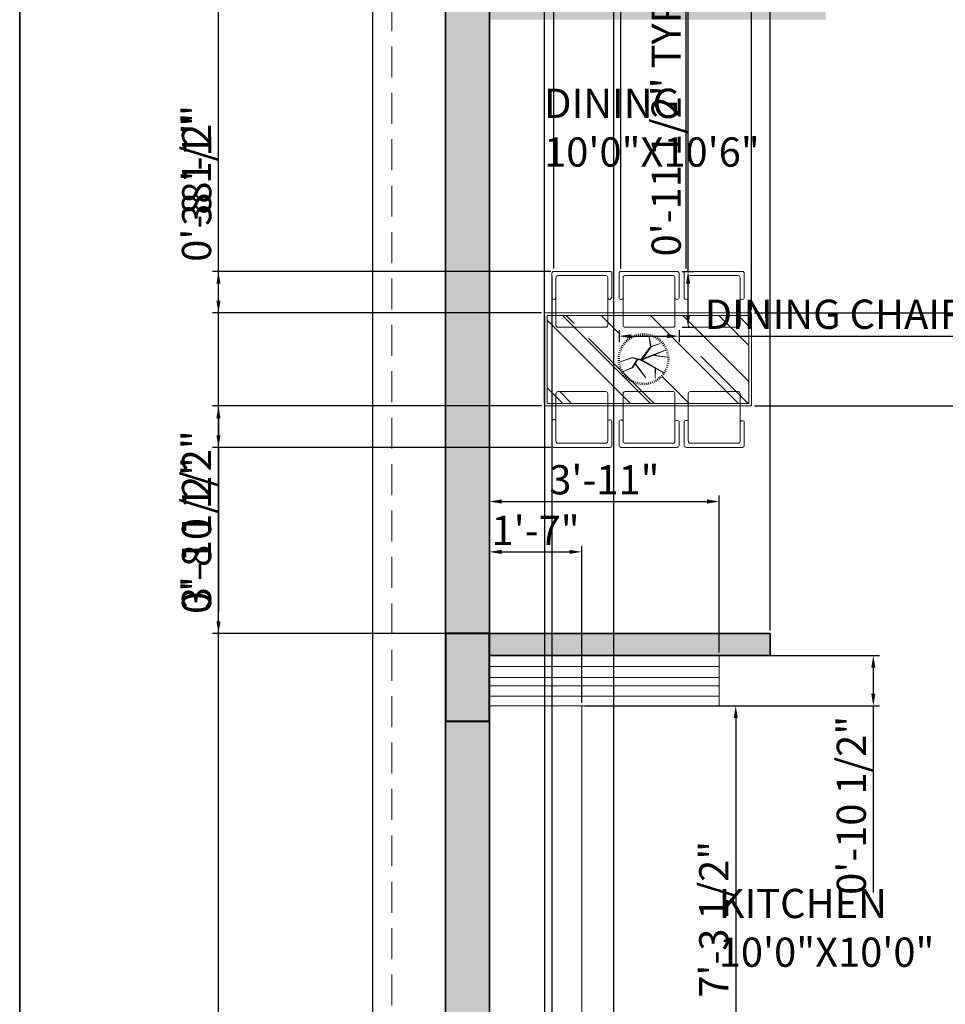
# Model space of a CAD drawing. Units: inches. Extents: x 2656 to 9931, y 1941 to 3068.
# Tile 2 of 46: x 2656 to 2846, y 2224 to 2426. Entities that reach past the tile are written whole.
import ezdxf

# ---------------------------------------------------------------- set-up
doc = ezdxf.new("R2010")
doc.units = ezdxf.units.IN
doc.linetypes.add('DASHED2', pattern=[9.525, 6.35, -3.175])
for name, color, linetype, lineweight in [('A-ANNO-DIMS', 2, 'Continuous', 18), ('A-ANNO-TTLB', 7, 'Continuous', 35), ('A-AREA-IDEN', 7, 'Continuous', 18), ('A-COLS', 7, 'Continuous', 40), ('A-COLS-PATT', 146, 'Continuous', 13), ('A-FLOR-CASE', 32, 'Continuous', 18), ('A-FLOR-OVHD', 252, 'DASHED2', 13), ('A-FURN', 8, 'Continuous', 13), ('A-FURN-PATT', 9, 'Continuous', 13), ('A-WALL', 7, 'Continuous', 35), ('A-WALL-PATT', 251, 'Continuous', 13), ('C-PROP', 7, 'Continuous', 25)]:
    doc.layers.add(name, color=color, linetype=linetype, lineweight=lineweight)
doc.styles.get("Standard").update_dxf_attribs({"font": 'arial.ttf'})
doc.dimstyles.new('ISO-25', dxfattribs={"dimtxt": 6, "dimasz": 2.5, "dimexe": 1.25, "dimexo": 0.625, "dimtad": 1, "dimdec": 0, "dimlunit": 3, "dimtxsty": 'Standard', "dimcen": 2.5, "dimadec": 0, "dimazin": 0, "dimtfac": 1, "dimtdec": 0, "dimtmove": 0, "dimatfit": 3, "dimfxl": 1, "dimarcsym": 0})

# ---------------------------------------------------------------- blocks, each defined once
blk = doc.blocks.new('CHAIR-DINING')
for p, q in [((-0.04, 6.08), (-0.04, 11.03)), ((0.34, 11.42), (11.9, 11.42)), ((0.81, 10.18), (0.81, 0.37)), ((1.19, 10.57), (11.05, 10.57)), ((11.43, 10.18), (11.43, 0.37)), ((12.28, 11.03), (12.28, 6.08)), ((0.34, 5.7), (0.43, 5.7)), ((11.82, 5.7), (11.9, 5.7)), ((1.19, -0.02), (11.05, -0.02))]:
    blk.add_line(p, q)
for centre, start, end in [((0.34, 11.03), 90, 180), ((1.19, 10.18), 90, 180), ((11.05, 10.18), 0, 90), ((11.9, 11.03), 0, 90), ((0.34, 6.08), 180, 270), ((0.43, 6.08), 270, 0), ((11.82, 6.08), 180, 270), ((11.9, 6.08), 270, 0), ((1.19, 0.37), 180, 270), ((11.05, 0.37), 270, 0)]:
    blk.add_arc(centre, 0.382, start, end)
blk = doc.blocks.new('*D61')
at = {"layer": 'A-ANNO-DIMS', "color": 0, "lineweight": -2, "transparency": 16777216}
for p, q in [((2778.76, 2362.36), (2778.76, 2359.89)), ((2781.26, 2361.14), (2788.58, 2361.14)), ((2791.08, 2362.36), (2791.08, 2359.89)), ((2791.08, 2361.14), (2905.16, 2361.14))]:
    blk.add_line(p, q, dxfattribs=at)
at = {"layer": 'A-ANNO-DIMS', "color": 0, "transparency": 16777216}
for points in [[(2781.26, 2361.55), (2781.26, 2360.72), (2778.76, 2361.14)], [(2788.58, 2361.55), (2788.58, 2360.72), (2791.08, 2361.14)]]:
    blk.add_solid(points, dxfattribs=at)
at = {"layer": 'Defpoints', "color": 0, "transparency": 16777216}
for p in [(2778.76, 2362.98), (2791.08, 2362.98), (2791.08, 2361.14)]:
    blk.add_point(p, dxfattribs=at)
at = {"layer": 'A-ANNO-DIMS', "color": 0, "transparency": 16777216, "insert": (2849.37, 2364.86), "char_height": 6, "attachment_point": 5}
blk.add_mtext('DINING CHAIR 1\'-0 1/2" TYP.', dxfattribs=at)
blk = doc.blocks.new('*D62')
at = {"layer": 'A-ANNO-DIMS', "color": 0, "lineweight": -2, "transparency": 16777216}
for p, q in [((2792.93, 2374.42), (2792.93, 2433.38)), ((2791.71, 2374.42), (2794.18, 2374.42)), ((2792.93, 2365.48), (2792.93, 2371.92)), ((2791.71, 2362.98), (2794.18, 2362.98))]:
    blk.add_line(p, q, dxfattribs=at)
at = {"layer": 'A-ANNO-DIMS', "color": 0, "transparency": 16777216}
for points in [[(2792.52, 2371.92), (2793.35, 2371.92), (2792.93, 2374.42)], [(2792.52, 2365.48), (2793.35, 2365.48), (2792.93, 2362.98)]]:
    blk.add_solid(points, dxfattribs=at)
at = {"layer": 'Defpoints', "color": 0, "transparency": 16777216}
for p in [(2791.08, 2374.42), (2792.93, 2374.42), (2791.08, 2362.98)]:
    blk.add_point(p, dxfattribs=at)
at = {"layer": 'A-ANNO-DIMS', "color": 0, "transparency": 16777216, "insert": (2789.21, 2405.15), "char_height": 6, "attachment_point": 5, "rotation": 90}
blk.add_mtext('0\'-11 1/2" TYP.', dxfattribs=at)
blk = doc.blocks.new('*D113')
at = {"layer": 'A-ANNO-DIMS', "color": 0, "lineweight": -2, "transparency": 16777216}
for p, q in [((2752.16, 2300.73), (2752.16, 2674.45)), ((2809.77, 2300.73), (2809.77, 2674.45)), ((2754.66, 2673.2), (2807.27, 2673.2))]:
    blk.add_line(p, q, dxfattribs=at)
at = {"layer": 'A-ANNO-DIMS', "color": 0, "transparency": 16777216}
for points in [[(2754.66, 2673.62), (2754.66, 2672.78), (2752.16, 2673.2)], [(2807.27, 2673.62), (2807.27, 2672.78), (2809.77, 2673.2)]]:
    blk.add_solid(points, dxfattribs=at)
at = {"layer": 'Defpoints', "color": 0, "transparency": 16777216}
for p in [(2809.77, 2673.2), (2752.16, 2300.1), (2809.77, 2300.1)]:
    blk.add_point(p, dxfattribs=at)
at = {"layer": 'A-ANNO-DIMS', "color": 0, "transparency": 16777216, "insert": (2780.96, 2676.93), "char_height": 6, "attachment_point": 5}
blk.add_mtext('4\'-9 1/2"', dxfattribs=at)
blk = doc.blocks.new('*D114')
at = {"layer": 'A-ANNO-DIMS', "color": 0, "lineweight": -2, "transparency": 16777216}
for p, q in [((2809.77, 2300.73), (2809.77, 2674.45)), ((2851.88, 2300.73), (2851.88, 2674.45)), ((2812.27, 2673.2), (2849.38, 2673.2))]:
    blk.add_line(p, q, dxfattribs=at)
at = {"layer": 'A-ANNO-DIMS', "color": 0, "transparency": 16777216}
for points in [[(2812.27, 2673.62), (2812.27, 2672.78), (2809.77, 2673.2)], [(2849.38, 2673.62), (2849.38, 2672.78), (2851.88, 2673.2)]]:
    blk.add_solid(points, dxfattribs=at)
at = {"layer": 'Defpoints', "color": 0, "transparency": 16777216}
for p in [(2851.88, 2673.2), (2809.77, 2300.1), (2851.88, 2300.1)]:
    blk.add_point(p, dxfattribs=at)
at = {"layer": 'A-ANNO-DIMS', "color": 0, "transparency": 16777216, "insert": (2830.82, 2676.89), "char_height": 6, "attachment_point": 5}
blk.add_mtext('3\'-6"', dxfattribs=at)
blk = doc.blocks.new('*D116')
at = {"layer": 'A-ANNO-DIMS', "color": 0, "lineweight": -2, "transparency": 16777216}
for p, q in [((2752.16, 2296.23), (2752.16, 2328.45)), ((2799.34, 2296.23), (2799.34, 2328.45)), ((2754.66, 2327.2), (2796.84, 2327.2))]:
    blk.add_line(p, q, dxfattribs=at)
at = {"layer": 'A-ANNO-DIMS', "color": 0, "transparency": 16777216}
for points in [[(2754.66, 2327.62), (2754.66, 2326.78), (2752.16, 2327.2)], [(2796.84, 2327.62), (2796.84, 2326.78), (2799.34, 2327.2)]]:
    blk.add_solid(points, dxfattribs=at)
at = {"layer": 'Defpoints', "color": 0, "transparency": 16777216}
for p in [(2799.34, 2327.2), (2752.16, 2295.6), (2799.34, 2295.6)]:
    blk.add_point(p, dxfattribs=at)
at = {"layer": 'A-ANNO-DIMS', "color": 0, "transparency": 16777216, "insert": (2775.75, 2330.89), "char_height": 6, "attachment_point": 5}
blk.add_mtext('3\'-11"', dxfattribs=at)
blk = doc.blocks.new('*D117')
at = {"layer": 'A-ANNO-DIMS', "color": 0, "lineweight": -2, "transparency": 16777216}
for p, q in [((2799.96, 2295.6), (2832.19, 2295.6)), ((2830.94, 2293.1), (2830.94, 2287.76)), ((2799.96, 2285.26), (2832.19, 2285.26)), ((2830.94, 2285.26), (2830.94, 2246.92))]:
    blk.add_line(p, q, dxfattribs=at)
at = {"layer": 'A-ANNO-DIMS', "color": 0, "transparency": 16777216}
for points in [[(2830.52, 2293.1), (2831.36, 2293.1), (2830.94, 2295.6)], [(2830.52, 2287.76), (2831.36, 2287.76), (2830.94, 2285.26)]]:
    blk.add_solid(points, dxfattribs=at)
at = {"layer": 'Defpoints', "color": 0, "transparency": 16777216}
for p in [(2799.34, 2295.6), (2799.34, 2285.26), (2830.94, 2285.26)]:
    blk.add_point(p, dxfattribs=at)
at = {"layer": 'A-ANNO-DIMS', "color": 0, "transparency": 16777216, "insert": (2827.21, 2264.84), "char_height": 6, "attachment_point": 5, "rotation": 90}
blk.add_mtext('0\'-10 1/2"', dxfattribs=at)
blk = doc.blocks.new('*D118')
at = {"layer": 'A-ANNO-DIMS', "color": 0, "lineweight": -2, "transparency": 16777216}
for p, q in [((2752.16, 2285.89), (2752.16, 2318.11)), ((2771.11, 2285.89), (2771.11, 2318.11)), ((2754.66, 2316.86), (2768.61, 2316.86))]:
    blk.add_line(p, q, dxfattribs=at)
at = {"layer": 'A-ANNO-DIMS', "color": 0, "transparency": 16777216}
for points in [[(2754.66, 2317.28), (2754.66, 2316.45), (2752.16, 2316.86)], [(2768.61, 2317.28), (2768.61, 2316.45), (2771.11, 2316.86)]]:
    blk.add_solid(points, dxfattribs=at)
at = {"layer": 'Defpoints', "color": 0, "transparency": 16777216}
for p in [(2771.11, 2316.86), (2752.16, 2285.26), (2771.11, 2285.26)]:
    blk.add_point(p, dxfattribs=at)
at = {"layer": 'A-ANNO-DIMS', "color": 0, "transparency": 16777216, "insert": (2761.63, 2320.5), "char_height": 6, "attachment_point": 5}
blk.add_mtext('1\'-7"', dxfattribs=at)
blk = doc.blocks.new('*D119')
at = {"layer": 'A-ANNO-DIMS', "color": 0, "lineweight": -2, "transparency": 16777216}
for p, q in [((2771.73, 2285.26), (2803.96, 2285.26)), ((2802.71, 2282.76), (2802.71, 2200.13)), ((2771.73, 2197.63), (2803.96, 2197.63))]:
    blk.add_line(p, q, dxfattribs=at)
at = {"layer": 'A-ANNO-DIMS', "color": 0, "transparency": 16777216}
for points in [[(2802.29, 2282.76), (2803.12, 2282.76), (2802.71, 2285.26)], [(2802.29, 2200.13), (2803.12, 2200.13), (2802.71, 2197.63)]]:
    blk.add_solid(points, dxfattribs=at)
at = {"layer": 'Defpoints', "color": 0, "transparency": 16777216}
for p in [(2771.11, 2285.26), (2771.11, 2197.63), (2802.71, 2197.63)]:
    blk.add_point(p, dxfattribs=at)
at = {"layer": 'A-ANNO-DIMS', "color": 0, "transparency": 16777216, "insert": (2798.98, 2241.45), "char_height": 6, "attachment_point": 5, "rotation": 90}
blk.add_mtext('7\'-3 1/2"', dxfattribs=at)
blk = doc.blocks.new('*D129')
at = {"layer": 'A-ANNO-DIMS', "color": 0, "lineweight": -2, "transparency": 16777216}
for p, q in [((2752.16, 2601.15), (2752.16, 2009.27)), ((2777.59, 2557.74), (2777.59, 2009.27)), ((2754.66, 2010.52), (2775.09, 2010.52)), ((2777.59, 2010.52), (2811.37, 2010.52))]:
    blk.add_line(p, q, dxfattribs=at)
at = {"layer": 'A-ANNO-DIMS', "color": 0, "transparency": 16777216}
for points in [[(2754.66, 2010.94), (2754.66, 2010.11), (2752.16, 2010.52)], [(2775.09, 2010.94), (2775.09, 2010.11), (2777.59, 2010.52)]]:
    blk.add_solid(points, dxfattribs=at)
at = {"layer": 'Defpoints', "color": 0, "transparency": 16777216}
for p in [(2752.16, 2601.77), (2777.59, 2558.37), (2777.59, 2010.52)]:
    blk.add_point(p, dxfattribs=at)
at = {"layer": 'A-ANNO-DIMS', "color": 0, "transparency": 16777216, "insert": (2795.73, 2014.25), "char_height": 6, "attachment_point": 5}
blk.add_mtext('2\'-1 1/2"', dxfattribs=at)
blk = doc.blocks.new('*D132')
at = {"layer": 'A-ANNO-DIMS', "color": 0, "lineweight": -2, "transparency": 16777216}
for p, q in [((2763.47, 2366.56), (2763.47, 2674.45)), ((2805.96, 2366.56), (2805.96, 2674.45)), ((2765.97, 2673.2), (2803.46, 2673.2))]:
    blk.add_line(p, q, dxfattribs=at)
at = {"layer": 'A-ANNO-DIMS', "color": 0, "transparency": 16777216}
for points in [[(2765.97, 2673.62), (2765.97, 2672.78), (2763.47, 2673.2)], [(2803.46, 2673.62), (2803.46, 2672.78), (2805.96, 2673.2)]]:
    blk.add_solid(points, dxfattribs=at)
at = {"layer": 'Defpoints', "color": 0, "transparency": 16777216}
for p in [(2805.96, 2673.2), (2763.47, 2365.93), (2805.96, 2365.93)]:
    blk.add_point(p, dxfattribs=at)
at = {"layer": 'A-ANNO-DIMS', "color": 0, "transparency": 16777216, "insert": (2784.72, 2676.93), "char_height": 6, "attachment_point": 5}
blk.add_mtext('3\'-6 1/2"', dxfattribs=at)
blk = doc.blocks.new('*D133')
at = {"layer": 'A-ANNO-DIMS', "color": 0, "lineweight": -2, "transparency": 16777216}
for p, q in [((2806.59, 2365.93), (3061.01, 2365.93)), ((3059.76, 2349.31), (3059.76, 2363.43)), ((2806.59, 2346.81), (3061.01, 2346.81))]:
    blk.add_line(p, q, dxfattribs=at)
at = {"layer": 'A-ANNO-DIMS', "color": 0, "transparency": 16777216}
for points in [[(3059.34, 2363.43), (3060.17, 2363.43), (3059.76, 2365.93)], [(3059.34, 2349.31), (3060.17, 2349.31), (3059.76, 2346.81)]]:
    blk.add_solid(points, dxfattribs=at)
at = {"layer": 'Defpoints', "color": 0, "transparency": 16777216}
for p in [(2805.96, 2365.93), (3059.76, 2365.93), (2805.96, 2346.81)]:
    blk.add_point(p, dxfattribs=at)
at = {"layer": 'A-ANNO-DIMS', "color": 0, "transparency": 16777216, "insert": (3056.12, 2356.37), "char_height": 6, "attachment_point": 5, "rotation": 90}
blk.add_mtext('1\'-7"', dxfattribs=at)
blk = doc.blocks.new('*D134')
at = {"layer": 'A-ANNO-DIMS', "color": 0, "lineweight": -2, "transparency": 16777216}
for p, q in [((2752.16, 2300.73), (2752.16, 2674.45)), ((2763.47, 2347.43), (2763.47, 2674.45)), ((2754.66, 2673.2), (2760.97, 2673.2)), ((2763.47, 2673.2), (2801.81, 2673.2))]:
    blk.add_line(p, q, dxfattribs=at)
at = {"layer": 'A-ANNO-DIMS', "color": 0, "transparency": 16777216}
for points in [[(2754.66, 2673.62), (2754.66, 2672.78), (2752.16, 2673.2)], [(2760.97, 2673.62), (2760.97, 2672.78), (2763.47, 2673.2)]]:
    blk.add_solid(points, dxfattribs=at)
at = {"layer": 'Defpoints', "color": 0, "transparency": 16777216}
for p in [(2763.47, 2673.2), (2763.47, 2346.81), (2752.16, 2300.1)]:
    blk.add_point(p, dxfattribs=at)
at = {"layer": 'A-ANNO-DIMS', "color": 0, "transparency": 16777216, "insert": (2783.89, 2676.93), "char_height": 6, "attachment_point": 5}
blk.add_mtext('0\'-11 1/2"', dxfattribs=at)
blk = doc.blocks.new('*D135')
at = {"layer": 'A-ANNO-DIMS', "color": 0, "lineweight": -2, "transparency": 16777216}
for p, q in [((2762.84, 2346.81), (2695.31, 2346.81)), ((2696.56, 2302.6), (2696.56, 2344.31)), ((2751.53, 2300.1), (2695.31, 2300.1))]:
    blk.add_line(p, q, dxfattribs=at)
at = {"layer": 'A-ANNO-DIMS', "color": 0, "transparency": 16777216}
for points in [[(2696.14, 2344.31), (2696.97, 2344.31), (2696.56, 2346.81)], [(2696.14, 2302.6), (2696.97, 2302.6), (2696.56, 2300.1)]]:
    blk.add_solid(points, dxfattribs=at)
at = {"layer": 'Defpoints', "color": 0, "transparency": 16777216}
for p in [(2696.56, 2346.81), (2763.47, 2346.81), (2752.16, 2300.1)]:
    blk.add_point(p, dxfattribs=at)
at = {"layer": 'A-ANNO-DIMS', "color": 0, "transparency": 16777216, "insert": (2692.83, 2323.45), "char_height": 6, "attachment_point": 5, "rotation": 90}
blk.add_mtext('3\'-10 1/2"', dxfattribs=at)
blk = doc.blocks.new('*D136')
at = {"layer": 'A-ANNO-DIMS', "color": 0, "lineweight": -2, "transparency": 16777216}
for p, q in [((2765.36, 2375.04), (2765.36, 2674.45)), ((2779.14, 2375.04), (2779.14, 2674.45)), ((2767.86, 2673.2), (2776.64, 2673.2)), ((2779.14, 2673.2), (2798.28, 2673.2))]:
    blk.add_line(p, q, dxfattribs=at)
at = {"layer": 'A-ANNO-DIMS', "color": 0, "transparency": 16777216}
for points in [[(2767.86, 2673.62), (2767.86, 2672.78), (2765.36, 2673.2)], [(2776.64, 2673.62), (2776.64, 2672.78), (2779.14, 2673.2)]]:
    blk.add_solid(points, dxfattribs=at)
at = {"layer": 'Defpoints', "color": 0, "transparency": 16777216}
for p in [(2779.14, 2673.2), (2765.36, 2374.42), (2779.14, 2374.42)]:
    blk.add_point(p, dxfattribs=at)
at = {"layer": 'A-ANNO-DIMS', "color": 0, "transparency": 16777216, "insert": (2789.96, 2676.84), "char_height": 6, "attachment_point": 5}
blk.add_mtext('1\'-2"', dxfattribs=at)
blk = doc.blocks.new('*D137')
at = {"layer": 'A-ANNO-DIMS', "color": 0, "lineweight": -2, "transparency": 16777216}
for p, q in [((2779.14, 2375.04), (2779.14, 2674.45)), ((2792.52, 2375.04), (2792.52, 2674.45)), ((2781.64, 2673.2), (2790.02, 2673.2)), ((2792.52, 2673.2), (2825.63, 2673.2))]:
    blk.add_line(p, q, dxfattribs=at)
at = {"layer": 'A-ANNO-DIMS', "color": 0, "transparency": 16777216}
for points in [[(2781.64, 2673.62), (2781.64, 2672.78), (2779.14, 2673.2)], [(2790.02, 2673.62), (2790.02, 2672.78), (2792.52, 2673.2)]]:
    blk.add_solid(points, dxfattribs=at)
at = {"layer": 'Defpoints', "color": 0, "transparency": 16777216}
for p in [(2792.52, 2673.2), (2779.14, 2374.42), (2792.52, 2374.42)]:
    blk.add_point(p, dxfattribs=at)
at = {"layer": 'A-ANNO-DIMS', "color": 0, "transparency": 16777216, "insert": (2810.32, 2676.93), "char_height": 6, "attachment_point": 5}
blk.add_mtext('1\'-1 1/2"', dxfattribs=at)
blk = doc.blocks.new('*D138')
at = {"layer": 'A-ANNO-DIMS', "color": 0, "lineweight": -2, "transparency": 16777216}
for p, q in [((2764.97, 2373.41), (2764.97, 2009.27)), ((2763.47, 2365.31), (2763.47, 2009.27)), ((2760.97, 2010.52), (2758.47, 2010.52)), ((2763.47, 2010.52), (2764.97, 2010.52)), ((2767.47, 2010.52), (2801.15, 2010.52))]:
    blk.add_line(p, q, dxfattribs=at)
at = {"layer": 'A-ANNO-DIMS', "color": 0, "transparency": 16777216}
for points in [[(2760.97, 2010.94), (2760.97, 2010.11), (2763.47, 2010.52)], [(2767.47, 2010.94), (2767.47, 2010.11), (2764.97, 2010.52)]]:
    blk.add_solid(points, dxfattribs=at)
at = {"layer": 'Defpoints', "color": 0, "transparency": 16777216}
for p in [(2764.97, 2374.03), (2763.47, 2365.93), (2764.97, 2010.52)]:
    blk.add_point(p, dxfattribs=at)
at = {"layer": 'A-ANNO-DIMS', "color": 0, "transparency": 16777216, "insert": (2785.56, 2014.25), "char_height": 6, "attachment_point": 5}
blk.add_mtext('0\'-1 1/2"', dxfattribs=at)
blk = doc.blocks.new('*D139')
at = {"layer": 'A-ANNO-DIMS', "color": 0, "lineweight": -2, "transparency": 16777216}
for p, q in [((2696.56, 2374.42), (2696.56, 2408.1)), ((2764.73, 2374.42), (2695.31, 2374.42)), ((2696.56, 2368.43), (2696.56, 2371.92)), ((2762.84, 2365.93), (2695.31, 2365.93))]:
    blk.add_line(p, q, dxfattribs=at)
at = {"layer": 'A-ANNO-DIMS', "color": 0, "transparency": 16777216}
for points in [[(2696.14, 2371.92), (2696.97, 2371.92), (2696.56, 2374.42)], [(2696.14, 2368.43), (2696.97, 2368.43), (2696.56, 2365.93)]]:
    blk.add_solid(points, dxfattribs=at)
at = {"layer": 'Defpoints', "color": 0, "transparency": 16777216}
for p in [(2696.56, 2374.42), (2765.36, 2374.42), (2763.47, 2365.93)]:
    blk.add_point(p, dxfattribs=at)
at = {"layer": 'A-ANNO-DIMS', "color": 0, "transparency": 16777216, "insert": (2692.83, 2392.51), "char_height": 6, "attachment_point": 5, "rotation": 90}
blk.add_mtext('0\'-8 1/2"', dxfattribs=at)
blk = doc.blocks.new('*D140')
at = {"layer": 'A-ANNO-DIMS', "color": 0, "lineweight": -2, "transparency": 16777216}
for p, q in [((2762.84, 2346.81), (2695.31, 2346.81)), ((2696.56, 2344.31), (2696.56, 2340.82)), ((2764.73, 2338.32), (2695.31, 2338.32)), ((2696.56, 2338.32), (2696.56, 2304.64))]:
    blk.add_line(p, q, dxfattribs=at)
at = {"layer": 'A-ANNO-DIMS', "color": 0, "transparency": 16777216}
for points in [[(2696.14, 2344.31), (2696.97, 2344.31), (2696.56, 2346.81)], [(2696.14, 2340.82), (2696.97, 2340.82), (2696.56, 2338.32)]]:
    blk.add_solid(points, dxfattribs=at)
at = {"layer": 'Defpoints', "color": 0, "transparency": 16777216}
for p in [(2763.47, 2346.81), (2696.56, 2338.32), (2765.36, 2338.32)]:
    blk.add_point(p, dxfattribs=at)
at = {"layer": 'A-ANNO-DIMS', "color": 0, "transparency": 16777216, "insert": (2692.83, 2320.23), "char_height": 6, "attachment_point": 5, "rotation": 90}
blk.add_mtext('0\'-8 1/2"', dxfattribs=at)
blk = doc.blocks.new('*D175')
at = {"layer": 'A-ANNO-DIMS', "color": 0, "lineweight": -2, "transparency": 16777216}
for p, q in [((2742.53, 2623.6), (2695.31, 2623.6)), ((2696.56, 2169.1), (2696.56, 2621.1)), ((2742.53, 2166.6), (2695.31, 2166.6))]:
    blk.add_line(p, q, dxfattribs=at)
at = {"layer": 'A-ANNO-DIMS', "color": 0, "transparency": 16777216}
for points in [[(2696.14, 2621.1), (2696.97, 2621.1), (2696.56, 2623.6)], [(2696.14, 2169.1), (2696.97, 2169.1), (2696.56, 2166.6)]]:
    blk.add_solid(points, dxfattribs=at)
at = {"layer": 'Defpoints', "color": 0, "transparency": 16777216}
for p in [(2696.56, 2623.6), (2743.16, 2623.6), (2743.16, 2166.6)]:
    blk.add_point(p, dxfattribs=at)
at = {"layer": 'A-ANNO-DIMS', "color": 0, "transparency": 16777216, "insert": (2692.87, 2395.1), "char_height": 6, "attachment_point": 5, "rotation": 90}
blk.add_mtext('38\'-1"', dxfattribs=at)

msp = doc.modelspace()

# ---------------------------------------------------------------- hatches: boundary and pattern name
at = {"layer": 'A-COLS-PATT'}
h = msp.add_hatch(color=256, dxfattribs=at)
h.dxf.hatch_style = 1
h.paths.add_polyline_path([(2752.16, 2623.6), (2743.16, 2623.6), (2743.16, 2605.6), (2752.16, 2605.6)])
h.paths.add_polyline_path([(2876.66, 2623.6), (2858.66, 2623.6), (2858.66, 2614.6), (2876.66, 2614.6)])
h.paths.add_polyline_path([(2998.16, 2623.6), (2989.16, 2623.6), (2989.16, 2614.6), (2989.16, 2605.6), (2998.16, 2605.6)])
h.paths.add_polyline_path([(2998.16, 2444.1), (2989.16, 2444.1), (2989.16, 2426.1), (2998.16, 2426.1)])
h.paths.add_polyline_path([(2876.66, 2444.1), (2867.66, 2444.1), (2867.66, 2426.1), (2876.66, 2426.1)])
h.paths.add_polyline_path([(2752.16, 2444.1), (2743.16, 2444.1), (2743.16, 2426.1), (2752.16, 2426.1)])
h.paths.add_polyline_path([(2752.16, 2300.1), (2743.16, 2300.1), (2743.16, 2282.1), (2752.16, 2282.1)])
h.paths.add_polyline_path([(2876.66, 2300.1), (2867.66, 2300.1), (2867.66, 2282.1), (2876.66, 2282.1)])
h.paths.add_polyline_path([(2998.16, 2300.1), (2989.16, 2300.1), (2989.16, 2282.1), (2998.16, 2282.1)])
h.paths.add_polyline_path([(2998.16, 2184.6), (2989.16, 2184.6), (2989.16, 2166.6), (2998.16, 2166.6)])
h.paths.add_polyline_path([(2876.66, 2175.6), (2858.66, 2175.6), (2858.66, 2166.6), (2876.66, 2166.6)])
h.paths.add_polyline_path([(2752.16, 2184.6), (2743.16, 2184.6), (2743.16, 2166.6), (2752.16, 2166.6)])
at = {"layer": 'A-FURN-PATT'}
h = msp.add_hatch(dxfattribs=at)
h.set_pattern_fill('AR-RROOF', color=256, scale=12.749297, angle=-45, style=0)
h.set_pattern_definition([(315, (3183.05, 3427.945), (28.84837, -10.81814), [191.2395, -25.4986, 63.7465, -12.7493]), (315, (3199.547, 3420.462), (2.975, 21.00522), [38.2479, -4.2073, 76.4958, -9.562]), (315, (3195.22, 3431.1), (52.91872, -40.83847), [101.9944, -17.849, 50.9972, -12.7493])])
h.paths.add_polyline_path([(2764, 2347.34), (2805.43, 2347.34), (2805.43, 2365.4), (2764, 2365.4)])
at = {"layer": 'A-WALL-PATT'}
h = msp.add_hatch(color=256, dxfattribs=at)
h.dxf.hatch_style = 1
h.paths.add_polyline_path([(2858.66, 2623.6), (2752.16, 2623.6), (2752.16, 2614.6), (2858.66, 2614.6)])
h.paths.add_polyline_path([(2893.09, 2623.6), (2876.66, 2623.6), (2876.66, 2614.6), (2893.09, 2614.6), (2893.09, 2619.1)])
h.paths.add_polyline_path([(2946.51, 2623.6), (2917.09, 2623.6), (2917.09, 2614.6), (2946.51, 2614.6), (2946.51, 2619.1)])
h.paths.add_polyline_path([(2989.16, 2623.6), (2970.51, 2623.6), (2970.51, 2614.6), (2989.16, 2614.6)])
h.paths.add_polyline_path([(2998.16, 2605.6), (2989.16, 2605.6), (2989.16, 2523.88), (2998.16, 2523.88)])
h.paths.add_polyline_path([(2935.16, 2614.6), (2930.66, 2614.6), (2930.66, 2554.6), (2876.66, 2554.6), (2876.66, 2565.34), (2872.16, 2565.34), (2872.16, 2444.1), (2876.66, 2444.1), (2876.66, 2550.1), (2946.47, 2550.1), (2946.47, 2554.6), (2935.16, 2554.6)])
h.paths.add_polyline_path([(2989.16, 2554.6), (2982.11, 2554.6), (2976.57, 2554.6), (2976.57, 2550.1), (2982.11, 2550.1), (2989.16, 2550.1)])
h.paths.add_polyline_path([(2876.66, 2614.6), (2872.16, 2614.6), (2872.16, 2595), (2876.66, 2595)], flags=0)
h.paths.add_polyline_path([(2752.16, 2605.6), (2743.16, 2605.6), (2743.16, 2544.03), (2752.16, 2544.03)])
h.paths.add_polyline_path([(2752.16, 2426.1), (2743.16, 2426.1), (2743.16, 2300.1), (2752.16, 2300.1)])
h.paths.add_polyline_path([(2821.13, 2430.6), (2752.16, 2430.6), (2752.16, 2426.1), (2821.13, 2426.1)])
h.paths.add_polyline_path([(2867.66, 2430.6), (2862.88, 2430.6), (2862.88, 2426.1), (2867.66, 2426.1)])
h.paths.add_polyline_path([(2752.16, 2484.03), (2747.66, 2484.03), (2743.16, 2484.03), (2743.16, 2444.1), (2752.16, 2444.1)])
h.paths.add_polyline_path([(2998.16, 2426.1), (2989.16, 2426.1), (2989.16, 2390.1), (2872.16, 2390.1), (2872.16, 2385.6), (2876.66, 2385.6), (2989.16, 2385.6), (2989.16, 2365.04), (2998.16, 2365.04)])
h.paths.add_polyline_path([(2998.16, 2463.88), (2993.66, 2463.88), (2989.16, 2463.88), (2989.16, 2444.1), (2998.16, 2444.1)])
h.paths.add_polyline_path([(2998.16, 2319.88), (2989.16, 2319.88), (2989.16, 2300.1), (2998.16, 2300.1)])
h.paths.add_polyline_path([(2998.16, 2282.1), (2989.16, 2282.1), (2989.16, 2253.6), (2982.06, 2253.6), (2982.06, 2249.1), (2989.16, 2249.1), (2998.16, 2249.1)])
h.paths.add_polyline_path([(2931.54, 2253.6), (2923.8, 2253.6), (2923.8, 2249.1), (2931.54, 2249.1)])
h.paths.add_polyline_path([(2876.66, 2282.1), (2872.16, 2282.1), (2872.16, 2184.6), (2872.16, 2175.6), (2876.66, 2175.6), (2876.66, 2249.1), (2888.32, 2249.1), (2888.32, 2251.35), (2888.32, 2253.6), (2876.66, 2253.6)])
h.paths.add_polyline_path([(2858.66, 2175.6), (2841.42, 2175.6), (2841.42, 2166.6), (2858.66, 2166.6)])
h.paths.add_polyline_path([(2785.06, 2171.1), (2785.06, 2175.6), (2752.16, 2175.6), (2752.16, 2166.6), (2785.06, 2166.6)])
h.paths.add_polyline_path([(2752.16, 2282.1), (2743.16, 2282.1), (2743.16, 2184.6), (2752.16, 2184.6)])
h.paths.add_polyline_path([(2809.77, 2300.1), (2752.16, 2300.1), (2752.16, 2295.6), (2809.77, 2295.6)])
h.paths.add_polyline_path([(2867.66, 2300.1), (2851.88, 2300.1), (2851.88, 2295.6), (2867.66, 2295.6)])

# ---------------------------------------------------------------- linework, layer by layer
at = {"layer": 'A-ANNO-TTLB'}
msp.add_lwpolyline([(2655.77, 3067.84), (3515.43, 3067.84), (3515.43, 1940.89), (2655.77, 1940.89)], close=True, dxfattribs=at)
at = {"layer": 'A-COLS'}
for p, q in [((2752.16, 2300.1), (2743.16, 2300.1)), ((2743.16, 2300.1), (2743.16, 2282.1)), ((2752.16, 2282.1), (2752.16, 2300.1)), ((2743.16, 2282.1), (2752.16, 2282.1))]:
    msp.add_line(p, q, dxfattribs=at)
at = {"layer": 'A-FLOR-CASE'}
for p, q in [((2799.34, 2285.26), (2799.34, 2295.6)), ((2799.34, 2293.34), (2752.16, 2293.34)), ((2799.34, 2291.1), (2752.16, 2291.1)), ((2799.34, 2289.4), (2752.16, 2289.4)), ((2799.34, 2287.26), (2752.16, 2287.26)), ((2799.34, 2285.26), (2799.34, 2287.26)), ((2752.16, 2285.26), (2799.34, 2285.26)), ((2771.11, 2285.26), (2771.11, 2197.63))]:
    msp.add_line(p, q, dxfattribs=at)
at = {"layer": 'A-FLOR-OVHD'}
msp.add_line((2732.16, 2166.6), (2732.16, 2637.6), dxfattribs=at)
at = {"layer": 'A-FURN'}
for p, q in [((2764.97, 2369.08), (2764.97, 2374.03)), ((2765.36, 2374.42), (2776.92, 2374.42)), ((2765.82, 2373.18), (2765.82, 2363.37)), ((2766.21, 2373.57), (2776.07, 2373.57)), ((2776.45, 2373.18), (2776.45, 2363.37)), ((2777.3, 2374.03), (2777.3, 2369.08)), ((2765.36, 2368.7), (2765.44, 2368.7)), ((2776.83, 2368.7), (2776.92, 2368.7)), ((2805.96, 2365.93), (2763.47, 2365.93)), ((2763.47, 2365.93), (2763.47, 2346.81)), ((2805.43, 2365.4), (2764, 2365.4)), ((2764, 2365.4), (2764, 2347.34)), ((2805.43, 2347.34), (2805.43, 2365.4)), ((2805.96, 2346.81), (2805.96, 2365.93)), ((2766.21, 2362.98), (2776.07, 2362.98)), ((2780.72, 2360.23), (2780.46, 2360.56)), ((2781.03, 2360.46), (2780.79, 2360.81)), ((2781.36, 2360.66), (2781.15, 2361.03)), ((2781.7, 2360.84), (2781.51, 2361.23)), ((2782.05, 2360.99), (2781.9, 2361.39)), ((2782.41, 2361.12), (2782.29, 2361.52)), ((2782.79, 2361.21), (2782.7, 2361.63)), ((2783.16, 2361.27), (2783.11, 2361.7)), ((2783.55, 2361.31), (2783.52, 2361.73)), ((2783.93, 2361.31), (2783.94, 2361.74)), ((2784.31, 2361.29), (2784.36, 2361.71)), ((2784.69, 2361.23), (2784.77, 2361.65)), ((2784.91, 2360.95), (2785.25, 2358.97)), ((2785.33, 2359.05), (2784.91, 2360.95)), ((2785.07, 2361.15), (2785.18, 2361.56)), ((2785.43, 2361.03), (2785.58, 2361.43)), ((2785.79, 2360.89), (2785.96, 2361.28)), ((2786.13, 2360.72), (2786.34, 2361.09)), ((2786.46, 2360.52), (2786.69, 2360.88)), ((2786.78, 2360.3), (2787.03, 2360.64)), ((2779.33, 2358.42), (2778.95, 2358.59)), ((2779.5, 2358.76), (2779.13, 2358.97)), ((2779.7, 2359.09), (2779.34, 2359.33)), ((2779.92, 2359.41), (2779.59, 2359.67)), ((2780.17, 2359.7), (2779.85, 2359.99)), ((2780.44, 2359.98), (2780.14, 2360.29)), ((2785.25, 2358.97), (2783.24, 2356.32)), ((2783.51, 2356.35), (2785.37, 2358.97)), ((2787.22, 2359.66), (2785.33, 2359.05)), ((2785.37, 2358.97), (2787.22, 2359.66)), ((2787.07, 2360.06), (2787.36, 2360.37)), ((2787.35, 2359.79), (2787.65, 2360.08)), ((2787.6, 2359.5), (2787.93, 2359.77)), ((2787.83, 2359.19), (2788.18, 2359.43)), ((2788.03, 2358.87), (2788.4, 2359.08)), ((2788.21, 2358.53), (2788.59, 2358.71)), ((2778.91, 2356.56), (2778.49, 2356.57)), ((2778.94, 2356.94), (2778.51, 2356.99)), ((2778.99, 2357.32), (2778.57, 2357.4)), ((2779.08, 2357.7), (2778.67, 2357.81)), ((2781.46, 2356.77), (2778.76, 2355.82)), ((2778.76, 2355.82), (2781.46, 2356.66)), ((2779.19, 2358.06), (2778.79, 2358.21)), ((2782.56, 2356.51), (2781.42, 2354.72)), ((2783.24, 2356.35), (2781.46, 2356.77)), ((2781.46, 2356.66), (2783.47, 2356.16)), ((2788.44, 2358.37), (2783.24, 2356.32)), ((2783.47, 2356.2), (2785.71, 2357.18)), ((2788.63, 2356.85), (2785.71, 2357.18)), ((2785.91, 2357.26), (2788.44, 2358.37)), ((2785.91, 2357.26), (2788.63, 2356.85)), ((2788.36, 2358.17), (2788.76, 2358.33)), ((2788.48, 2357.81), (2788.89, 2357.93)), ((2788.58, 2357.44), (2788.99, 2357.53)), ((2788.64, 2357.06), (2789.06, 2357.12)), ((2788.68, 2356.68), (2789.1, 2356.7)), ((2778.92, 2356.18), (2778.49, 2356.16)), ((2778.95, 2355.8), (2778.53, 2355.74)), ((2779.01, 2355.42), (2778.6, 2355.33)), ((2779.11, 2355.05), (2778.7, 2354.92)), ((2779.23, 2354.68), (2778.83, 2354.53)), ((2781.42, 2354.72), (2779.6, 2353.89)), ((2779.6, 2353.89), (2781.53, 2354.64)), ((2781.53, 2354.64), (2782.59, 2356.39)), ((2784.26, 2352.56), (2782.03, 2355.56)), ((2782.14, 2355.56), (2784.26, 2352.56)), ((2786.16, 2354.59), (2783.28, 2356.16)), ((2783.51, 2356.2), (2787.95, 2353.62)), ((2786.16, 2352.52), (2786.16, 2354.59)), ((2786.25, 2354.54), (2786.16, 2352.52)), ((2787.95, 2353.62), (2786.25, 2354.54)), ((2788.4, 2354.79), (2788.8, 2354.65)), ((2788.52, 2355.16), (2788.93, 2355.05)), ((2788.6, 2355.53), (2789.02, 2355.45)), ((2788.66, 2355.91), (2789.08, 2355.87)), ((2788.68, 2356.29), (2789.11, 2356.28)), ((2779.38, 2354.33), (2779, 2354.15)), ((2779.56, 2353.99), (2779.19, 2353.78)), ((2779.77, 2353.66), (2779.42, 2353.42)), ((2779.99, 2353.36), (2779.66, 2353.09)), ((2780.25, 2353.07), (2779.94, 2352.78)), ((2780.52, 2352.8), (2780.24, 2352.48)), ((2780.82, 2352.55), (2780.56, 2352.22)), ((2786.87, 2352.63), (2787.13, 2352.3)), ((2787.16, 2352.88), (2787.45, 2352.57)), ((2787.42, 2353.15), (2787.74, 2352.87)), ((2787.67, 2353.45), (2788.01, 2353.19)), ((2787.89, 2353.76), (2788.25, 2353.53)), ((2788.09, 2354.09), (2788.46, 2353.89)), ((2788.26, 2354.44), (2788.65, 2354.26)), ((2781.13, 2352.33), (2780.9, 2351.98)), ((2781.46, 2352.14), (2781.26, 2351.76)), ((2781.8, 2351.97), (2781.63, 2351.58)), ((2782.16, 2351.82), (2782.02, 2351.42)), ((2782.53, 2351.71), (2782.42, 2351.3)), ((2782.9, 2351.62), (2782.82, 2351.21)), ((2783.28, 2351.57), (2783.24, 2351.15)), ((2783.66, 2351.54), (2783.65, 2351.12)), ((2784.05, 2351.55), (2784.07, 2351.12)), ((2784.43, 2351.58), (2784.48, 2351.16)), ((2784.81, 2351.65), (2784.9, 2351.23)), ((2785.18, 2351.74), (2785.3, 2351.33)), ((2785.54, 2351.86), (2785.69, 2351.47)), ((2785.9, 2352.01), (2786.08, 2351.63)), ((2786.24, 2352.19), (2786.45, 2351.82)), ((2786.56, 2352.4), (2786.8, 2352.05)), ((2765.82, 2349.37), (2765.82, 2339.56)), ((2766.21, 2349.76), (2776.07, 2349.76)), ((2776.45, 2339.56), (2776.45, 2349.37)), ((2779.61, 2349.37), (2779.61, 2339.56)), ((2779.99, 2349.76), (2789.85, 2349.76)), ((2790.23, 2339.56), (2790.23, 2349.37)), ((2792.98, 2339.56), (2792.98, 2349.37)), ((2803.23, 2349.76), (2793.37, 2349.76)), ((2803.61, 2349.37), (2803.61, 2339.56)), ((2763.47, 2346.81), (2805.96, 2346.81)), ((2764, 2347.34), (2805.43, 2347.34)), ((2764.97, 2343.66), (2764.97, 2338.71)), ((2765.36, 2344.04), (2765.44, 2344.04)), ((2776.83, 2343.96), (2776.92, 2343.96)), ((2777.3, 2338.71), (2777.3, 2343.66)), ((2778.76, 2343.66), (2778.76, 2338.71)), ((2779.14, 2343.95), (2779.23, 2343.95)), ((2790.62, 2343.87), (2790.7, 2343.87)), ((2791.08, 2338.71), (2791.08, 2343.66)), ((2792.13, 2338.71), (2792.13, 2343.66)), ((2792.6, 2343.86), (2792.52, 2343.86)), ((2804.08, 2343.78), (2803.99, 2343.78)), ((2804.46, 2343.66), (2804.46, 2338.71)), ((2765.36, 2338.32), (2776.92, 2338.32)), ((2766.21, 2339.17), (2776.07, 2339.17)), ((2779.14, 2338.32), (2790.7, 2338.32)), ((2779.99, 2339.17), (2789.85, 2339.17)), ((2804.08, 2338.32), (2792.52, 2338.32)), ((2803.23, 2339.17), (2793.37, 2339.17))]:
    msp.add_line(p, q, dxfattribs=at)
for centre, start, end in [((2765.36, 2374.03), 90, 180), ((2766.21, 2373.18), 90, 180), ((2776.07, 2373.18), 0, 90), ((2776.92, 2374.03), 0, 90), ((2765.36, 2369.08), 180, 0.104), ((2776.83, 2369.08), 180, 0.104), ((2766.21, 2363.37), 180, 270), ((2776.07, 2363.37), 270, 0), ((2766.21, 2349.37), 90, 180), ((2776.07, 2349.37), 0, 90), ((2779.99, 2349.37), 90, 180), ((2789.85, 2349.37), 0, 90), ((2793.37, 2349.37), 90, 180), ((2803.23, 2349.37), 0, 90), ((2765.36, 2343.65), 89.6202, 179.6202), ((2765.44, 2343.65), 359.6202, 89.6202), ((2776.83, 2343.58), 89.6202, 179.6202), ((2776.92, 2343.58), 359.6202, 89.6202), ((2779.14, 2343.56), 89.6202, 179.6202), ((2779.23, 2343.56), 359.6202, 89.6202), ((2790.62, 2343.49), 89.6202, 179.6202), ((2790.7, 2343.49), 359.6202, 89.6202), ((2792.52, 2343.47), 89.6202, 179.6202), ((2792.6, 2343.47), 359.6202, 89.6202), ((2803.99, 2343.4), 89.6202, 179.6202), ((2804.07, 2343.4), 359.6202, 89.6202), ((2765.36, 2338.71), 180, 270), ((2766.21, 2339.56), 180, 270), ((2776.07, 2339.56), 270, 0), ((2776.92, 2338.71), 270, 0), ((2779.14, 2338.71), 180, 270), ((2779.99, 2339.56), 180, 270), ((2789.85, 2339.56), 270, 0), ((2790.7, 2338.71), 270, 0), ((2792.52, 2338.71), 180, 270), ((2793.37, 2339.56), 180, 270), ((2803.23, 2339.56), 270, 0), ((2804.08, 2338.71), 270, 0)]:
    msp.add_arc(centre, 0.382, start, end, dxfattribs=at)
at = {"layer": 'A-WALL'}
for p, q in [((2743.16, 2623.6), (2743.16, 2166.6)), ((2752.16, 2614.6), (2752.16, 2166.6)), ((2752.16, 2300.1), (2809.77, 2300.1)), ((2809.77, 2300.1), (2809.77, 2295.6)), ((2752.16, 2295.6), (2809.77, 2295.6))]:
    msp.add_line(p, q, dxfattribs=at)
at = {"layer": 'C-PROP'}
msp.add_line((2728.16, 2641.6), (2728.16, 2086.1), dxfattribs=at)

# ---------------------------------------------------------------- block references
at = {"layer": 'A-FURN'}
for p in [(2778.8, 2363), (2792.17, 2363)]:
    msp.add_blockref('CHAIR-DINING', p, dxfattribs=at)

# ---------------------------------------------------------------- texts
at = {"layer": 'A-AREA-IDEN', "char_height": 6, "attachment_point": 1}
for s, insert in [('DINING\\P10\'0"X10\'6"', (2763.38, 2411.94)), ('KITCHEN \\P10\'0"X10\'0"', (2799.22, 2247.7))]:
    msp.add_mtext_dynamic_manual_height_columns(s, width=137.4726, gutter_width=12.5, heights=[0], dxfattribs=dict(at, insert=insert))

# ---------------------------------------------------------------- dimensions: what is measured, and where the dimension line sits
at = {"layer": 'A-ANNO-DIMS'}
for base, p1, p2, picture, middle in [((2809.77, 2673.2), (2752.16, 2300.1), (2809.77, 2300.1), '*D113', (2780.96, 2676.93)), ((2763.47, 2673.2), (2752.16, 2300.1), (2763.47, 2346.81), '*D134', (2783.89, 2676.93)), ((2805.96, 2673.2), (2763.47, 2365.93), (2805.96, 2365.93), '*D132', (2784.72, 2676.93)), ((2792.52, 2673.2), (2779.14, 2374.42), (2792.52, 2374.42), '*D137', (2810.32, 2676.93)), ((2779.14, 2673.2), (2765.36, 2374.42), (2779.14, 2374.42), '*D136', (2789.96, 2676.84)), ((2851.88, 2673.2), (2809.77, 2300.1), (2851.88, 2300.1), '*D114', (2830.82, 2676.89)), ((2777.59, 2010.52), (2752.16, 2601.77), (2777.59, 2558.37), '*D129', (2795.73, 2014.25)), ((2764.97, 2010.52), (2763.47, 2365.93), (2764.97, 2374.03), '*D138', (2785.56, 2014.25)), ((2799.34, 2327.2), (2752.16, 2295.6), (2799.34, 2295.6), '*D116', (2775.75, 2330.89)), ((2771.108, 2316.8622), (2752.1573, 2285.2622), (2771.108, 2285.2622), '*D118', (2761.6327, 2320.4995))]:
    dim = msp.add_linear_dim(base=base, p1=p1, p2=p2, dimstyle='ISO-25', override={"dimdec": 1, "dimlfac": 1, "dimrnd": 0, "dimzin": 1, "dimdsep": 46, "dimlunit": 4, "dimfrac": 2}, dxfattribs=at)
    dim.commit()
    dim.dimension.update_dxf_attribs({"geometry": picture, "text_midpoint": middle})
for base, p1, p2, angle, picture, middle in [((2696.56, 2623.6), (2743.16, 2166.6), (2743.16, 2623.6), 90, '*D175', (2692.87, 2395.1)), ((2696.56, 2374.42), (2763.47, 2365.93), (2765.36, 2374.42), 90, '*D139', (2692.83, 2392.51)), ((3059.76, 2365.93), (2805.96, 2346.81), (2805.96, 2365.93), 90, '*D133', (3056.12, 2356.37)), ((2696.56, 2346.81), (2752.16, 2300.1), (2763.47, 2346.81), 90, '*D135', (2692.83, 2323.45)), ((2696.56, 2338.32), (2763.47, 2346.81), (2765.36, 2338.32), 90, '*D140', (2692.83, 2320.23)), ((2830.94, 2285.26), (2799.34, 2295.6), (2799.34, 2285.26), 270, '*D117', (2827.21, 2264.84)), ((2802.71, 2197.63), (2771.11, 2285.26), (2771.11, 2197.63), 270, '*D119', (2798.98, 2241.45))]:
    dim = msp.add_linear_dim(base=base, p1=p1, p2=p2, angle=angle, dimstyle='ISO-25', override={"dimdec": 1, "dimlfac": 1, "dimrnd": 0, "dimzin": 1, "dimdsep": 46, "dimlunit": 4, "dimfrac": 2}, dxfattribs=at)
    dim.commit()
    dim.dimension.update_dxf_attribs({"geometry": picture, "text_midpoint": middle})
dim = msp.add_linear_dim(base=(2792.93, 2374.42), p1=(2791.08, 2362.98), p2=(2791.08, 2374.42), angle=90, text='<> TYP.', dimstyle='ISO-25', override={"dimdec": 1, "dimlfac": 1, "dimrnd": 0, "dimzin": 1, "dimdsep": 46, "dimlunit": 4, "dimfrac": 2}, dxfattribs=at)
dim.commit()
dim.dimension.update_dxf_attribs({"geometry": '*D62', "text_midpoint": (2789.21, 2405.15)})
dim = msp.add_linear_dim(base=(2791.08, 2361.14), p1=(2778.76, 2362.98), p2=(2791.08, 2362.98), text='DINING CHAIR <> TYP.', dimstyle='ISO-25', override={"dimdec": 1, "dimlfac": 1, "dimrnd": 0, "dimzin": 1, "dimdsep": 46, "dimlunit": 4, "dimfrac": 2}, dxfattribs=at)
dim.commit()
dim.dimension.update_dxf_attribs({"geometry": '*D61', "text_midpoint": (2849.37, 2364.86)})

doc.saveas('drawing.dxf')
